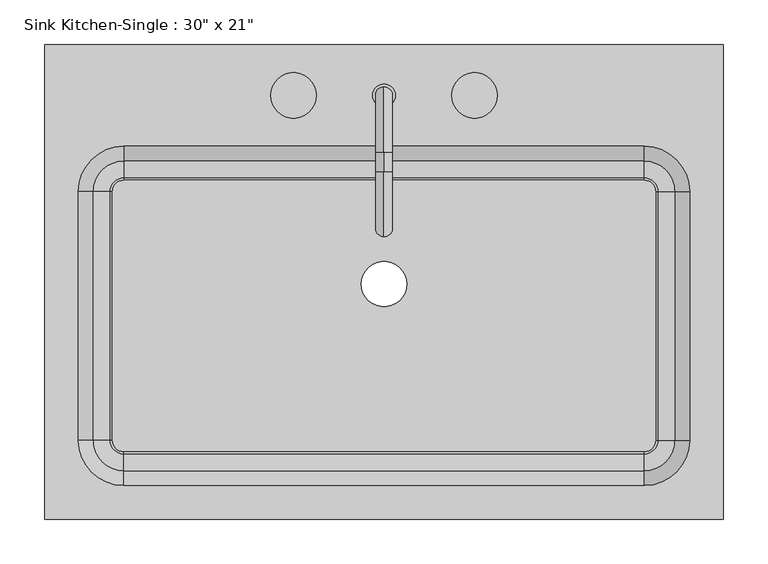
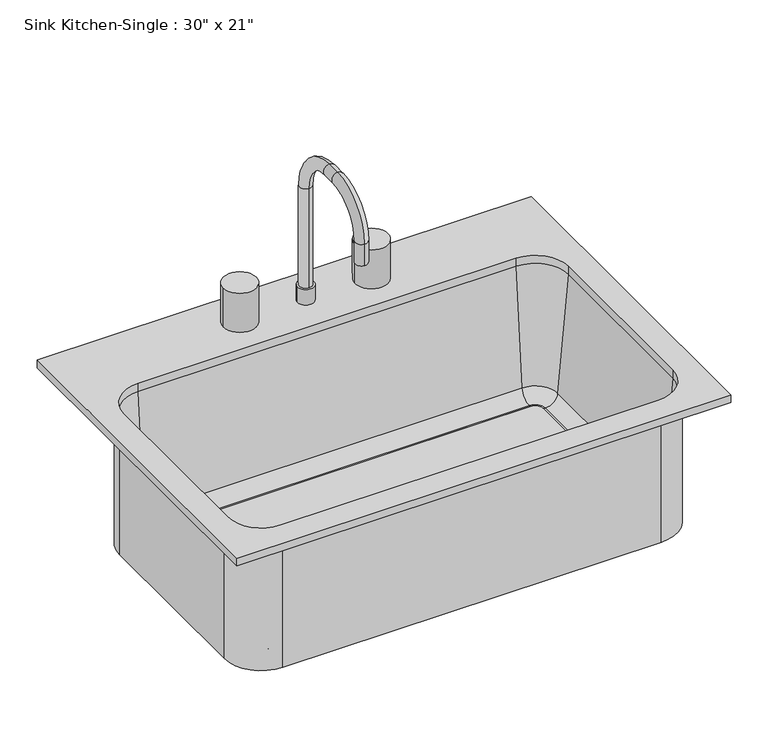
"""IFC4 building model written with IfcOpenShell, lengths in millimetres: flow terminal geometry."""

from ifc_helpers import new_model, si_unit, point, frame, frame_2d, origin, place, context, project, spatial, polyline, circle_curve, ellipse_curve, trimmed, segment, composite_curve, outline, extrude, source, transform, mapped, element, save
from ifc_brep_helpers import plane_surface, cylinder_surface, revolved_surface, advanced_brep


def flow_terminal_4d548711(model_context):
    return source(origin(), model_context, "Body", "SolidModel", [
        extrude(outline(composite_curve([segment(trimmed(circle_curve(frame_2d((307.7892406, 103.9454011)), 12.7), [point((307.7892406, 116.6454011))], [point((320.4892406, 103.9454011))], False, "CARTESIAN"), True, "CONTINUOUS"), segment(polyline([(320.4892406, 103.9454011), (320.4892406, -175.4545989)]), True, "CONTINUOUS"), segment(trimmed(circle_curve(frame_2d((307.7892406, -175.4545989)), 12.7), [point((320.4892406, -175.4545989))], [point((307.7892406, -188.1545989))], False, "CARTESIAN"), True, "CONTINUOUS"), segment(polyline([(307.7892406, -188.1545989), (-276.4107594, -188.1545989)]), True, "CONTINUOUS"), segment(trimmed(circle_curve(frame_2d((-276.4107594, -175.4545989)), 12.7), [point((-276.4107594, -188.1545989))], [point((-289.1107594, -175.4545989))], False, "CARTESIAN"), True, "CONTINUOUS"), segment(polyline([(-289.1107594, -175.4545989), (-289.1107594, 103.9454011)]), True, "CONTINUOUS"), segment(trimmed(circle_curve(frame_2d((-276.4107594, 103.9454011)), 12.7), [point((-289.1107594, 103.9454011))], [point((-276.4107594, 116.6454011))], False, "CARTESIAN"), True, "CONTINUOUS"), segment(polyline([(-276.4107594, 116.6454011), (307.7892406, 116.6454011)]), True, "CONTINUOUS")], self_intersect=False), holes=[composite_curve([segment(trimmed(circle_curve(frame_2d((15.6892406, 0.0)), 25.4), [point((-9.7107594, 0.0))], [point((41.0892406, 0.0))], True, "CARTESIAN"), True, "CONTINUOUS"), segment(trimmed(circle_curve(frame_2d((15.6892406, 0.0)), 25.4), [point((41.0892406, 0.0))], [point((-9.7107594, 0.0))], True, "CARTESIAN"), True, "CONTINUOUS")], self_intersect=False)]), frame((0.0, 0.0, 698.5), z_axis=(0.0, 0.0, 1.0), x_axis=(1.0, 0.0, 0.0)), (0.0, 0.0, 1.0), 9.525),
        extrude(outline(composite_curve([segment(trimmed(circle_curve(frame_2d((-85.9107594, 211.8954011)), 25.4), [point((-111.3107594, 211.8954011))], [point((-60.5107594, 211.8954011))], False, "CARTESIAN"), True, "CONTINUOUS"), segment(trimmed(circle_curve(frame_2d((-85.9107594, 211.8954011)), 25.4), [point((-60.5107594, 211.8954011))], [point((-111.3107594, 211.8954011))], False, "CARTESIAN"), True, "CONTINUOUS")], self_intersect=False)), frame((0.0, 0.0, 927.1), z_axis=(0.0, 0.0, 1.0), x_axis=(1.0, 0.0, 0.0)), (0.0, 0.0, 1.0), 63.5),
        extrude(outline(composite_curve([segment(trimmed(circle_curve(frame_2d((117.2892406, 211.8954011)), 25.4), [point((91.8892406, 211.8954011))], [point((142.6892406, 211.8954011))], False, "CARTESIAN"), True, "CONTINUOUS"), segment(trimmed(circle_curve(frame_2d((117.2892406, 211.8954011)), 25.4), [point((142.6892406, 211.8954011))], [point((91.8892406, 211.8954011))], False, "CARTESIAN"), True, "CONTINUOUS")], self_intersect=False)), frame((0.0, 0.0, 927.1), z_axis=(0.0, 0.0, 1.0), x_axis=(1.0, 0.0, 0.0)), (0.0, 0.0, 1.0), 63.5),
        advanced_brep(
        [(2.9892406, 211.8954011, 927.1), (28.3892406, 211.8954011, 927.1), (15.6892406, 221.4204011, 1114.425), (15.6892406, 202.3704011, 1114.425), (15.6892406, 202.3704011, 952.5), (15.6892406, 221.4204011, 952.5), (15.6892406, 148.3954011, 1187.45), (15.6892406, 148.3954011, 1168.4), (15.6892406, 126.1704011, 1187.45), (15.6892406, 126.1704011, 1168.4), (15.6892406, 53.1454011, 1114.425), (15.6892406, 72.1954011, 1114.425), (15.6892406, 53.1454011, 1079.5), (15.6892406, 72.1954011, 1079.5), (2.9892406, 211.8954011, 952.5), (28.3892406, 211.8954011, 952.5)],
        [
            (0, 1, circle_curve(frame((15.6892406, 211.8954011, 927.1), z_axis=(0.0, 0.0, -1.0), x_axis=(1.0, 0.0, 0.0)), 12.7)),
            (1, 0, circle_curve(frame((15.6892406, 211.8954011, 927.1), z_axis=(0.0, 0.0, -1.0), x_axis=(1.0, 0.0, 0.0)), 12.7)),
            (2, 3, circle_curve(frame((15.6892406, 211.8954011, 1114.425), z_axis=(0.0, 0.0, -1.0), x_axis=(0.0, -1.0, 0.0)), 9.525)),
            (3, 4),
            (4, 5, circle_curve(frame((15.6892406, 211.8954011, 952.5), z_axis=(0.0, 0.0, 1.0), x_axis=(0.0, -1.0, 0.0)), 9.525)),
            (5, 2),
            (3, 2, circle_curve(frame((15.6892406, 211.8954011, 1114.425), z_axis=(0.0, 0.0, -1.0), x_axis=(0.0, -1.0, 0.0)), 9.525)),
            (5, 4, circle_curve(frame((15.6892406, 211.8954011, 952.5), z_axis=(0.0, 0.0, 1.0), x_axis=(0.0, -1.0, 0.0)), 9.525)),
            (2, 6, circle_curve(frame((15.6892406, 148.3954011, 1114.425), z_axis=(1.0, 0.0, 0.0), x_axis=(0.0, 1.0, 0.0)), 73.025)),
            (6, 7, circle_curve(frame((15.6892406, 148.3954011, 1177.925), z_axis=(0.0, 1.0, 0.0), x_axis=(0.0, 0.0, -1.0)), 9.525)),
            (7, 3, circle_curve(frame((15.6892406, 148.3954011, 1114.425), z_axis=(-1.0, 0.0, 0.0), x_axis=(0.0, 1.0, 0.0)), 53.975)),
            (7, 6, circle_curve(frame((15.6892406, 148.3954011, 1177.925), z_axis=(0.0, 1.0, 0.0), x_axis=(0.0, 0.0, -1.0)), 9.525)),
            (6, 8),
            (8, 9, circle_curve(frame((15.6892406, 126.1704011, 1177.925), z_axis=(0.0, 1.0, 0.0), x_axis=(0.0, 0.0, -1.0)), 9.525)),
            (9, 7),
            (9, 8, circle_curve(frame((15.6892406, 126.1704011, 1177.925), z_axis=(0.0, 1.0, 0.0), x_axis=(0.0, 0.0, -1.0)), 9.525)),
            (8, 10, circle_curve(frame((15.6892406, 126.1704011, 1114.425), z_axis=(1.0, 0.0, 0.0), x_axis=(0.0, 0.0, 1.0)), 73.025)),
            (10, 11, circle_curve(frame((15.6892406, 62.6704011, 1114.425), z_axis=(0.0, 0.0, 1.0), x_axis=(0.0, 1.0, 0.0)), 9.525)),
            (11, 9, circle_curve(frame((15.6892406, 126.1704011, 1114.425), z_axis=(-1.0, 0.0, 0.0), x_axis=(0.0, 0.0, 1.0)), 53.975)),
            (11, 10, circle_curve(frame((15.6892406, 62.6704011, 1114.425), z_axis=(0.0, 0.0, 1.0), x_axis=(0.0, 1.0, 0.0)), 9.525)),
            (12, 13, circle_curve(frame((15.6892406, 62.6704011, 1079.5), z_axis=(0.0, 0.0, -1.0), x_axis=(0.0, 1.0, 0.0)), 9.525)),
            (13, 12, circle_curve(frame((15.6892406, 62.6704011, 1079.5), z_axis=(0.0, 0.0, -1.0), x_axis=(0.0, 1.0, 0.0)), 9.525)),
            (10, 12),
            (13, 11),
            (14, 15, circle_curve(frame((15.6892406, 211.8954011, 952.5), z_axis=(0.0, 0.0, 1.0), x_axis=(1.0, 0.0, 0.0)), 12.7)),
            (15, 14, circle_curve(frame((15.6892406, 211.8954011, 952.5), z_axis=(0.0, 0.0, 1.0), x_axis=(1.0, 0.0, 0.0)), 12.7)),
            (14, 0),
            (1, 15),
        ],
        [
            plane_surface(frame((15.6892406, 202.3704011, 927.1), z_axis=(0.0, 0.0, -1.0), x_axis=(1.0, 0.0, 0.0))),
            cylinder_surface(frame((15.6892406, 211.8954011, 927.1), z_axis=(0.0, 0.0, -1.0), x_axis=(0.0, -1.0, 0.0)), 9.525),
            revolved_surface(trimmed(ellipse_curve(frame((15.6892406, 211.8954011, 1114.425), z_axis=(0.0, 0.0, -1.0), x_axis=(0.0, -1.0, 0.0)), 9.525, 9.525), [point((15.6892406, 221.4204011, 1114.425))], [point((15.6892406, 202.3704011, 1114.425))], True, "CARTESIAN"), (15.6892406, 148.3954011, 1114.425), (1.0, 0.0, 0.0)),
            revolved_surface(trimmed(ellipse_curve(frame((15.6892406, 211.8954011, 1114.425), z_axis=(0.0, 0.0, -1.0), x_axis=(0.0, -1.0, 0.0)), 9.525, 9.525), [point((15.6892406, 202.3704011, 1114.425))], [point((15.6892406, 221.4204011, 1114.425))], True, "CARTESIAN"), (15.6892406, 148.3954011, 1114.425), (1.0, 0.0, 0.0)),
            cylinder_surface(frame((15.6892406, 148.3954011, 1177.925), z_axis=(0.0, 1.0, 0.0), x_axis=(0.0, 0.0, -1.0)), 9.525),
            revolved_surface(trimmed(ellipse_curve(frame((15.6892406, 126.1704011, 1177.925), z_axis=(0.0, 1.0, 0.0), x_axis=(0.0, 0.0, -1.0)), 9.525, 9.525), [point((15.6892406, 126.1704011, 1187.45))], [point((15.6892406, 126.1704011, 1168.4))], True, "CARTESIAN"), (15.6892406, 126.1704011, 1114.425), (1.0, 0.0, 0.0)),
            revolved_surface(trimmed(ellipse_curve(frame((15.6892406, 126.1704011, 1177.925), z_axis=(0.0, 1.0, 0.0), x_axis=(0.0, 0.0, -1.0)), 9.525, 9.525), [point((15.6892406, 126.1704011, 1168.4))], [point((15.6892406, 126.1704011, 1187.45))], True, "CARTESIAN"), (15.6892406, 126.1704011, 1114.425), (1.0, 0.0, 0.0)),
            plane_surface(frame((15.6892406, 53.1454011, 1079.5), z_axis=(0.0, 0.0, -1.0), x_axis=(-1.0, 0.0, 0.0))),
            cylinder_surface(frame((15.6892406, 62.6704011, 1114.425), z_axis=(0.0, 0.0, 1.0), x_axis=(0.0, 1.0, 0.0)), 9.525),
            plane_surface(frame((28.3892406, 211.8954011, 952.5), z_axis=(0.0, 0.0, 1.0), x_axis=(0.0, 1.0, 0.0))),
            cylinder_surface(frame((15.6892406, 211.8954011, 927.1), z_axis=(0.0, 0.0, 1.0), x_axis=(1.0, 0.0, 0.0)), 12.7),
        ],
        [
            (0, [[1, 2]]),
            (1, [[3, 4, 5, 6]]),
            (1, [[7, -6, 8, -4]]),
            (2, [[-3, 9, 10, 11]]),
            (3, [[-7, -11, 12, -9]]),
            (4, [[-10, 13, 14, 15]]),
            (4, [[-12, -15, 16, -13]]),
            (5, [[-14, 17, 18, 19]]),
            (6, [[-16, -19, 20, -17]]),
            (7, [[21, 22]]),
            (8, [[-18, 23, -22, 24]]),
            (8, [[-20, -24, -21, -23]]),
            (9, [[25, 26], [-5, -8]]),
            (10, [[-25, 27, -2, 28]]),
            (10, [[-26, -28, -1, -27]]),
        ],
    ),
        advanced_brep(
        [(396.6892406, 269.0454011, 927.1), (-365.3107594, 269.0454011, 927.1), (-365.3107594, -264.3545989, 927.1), (396.6892406, -264.3545989, 927.1), (307.7892406, 154.7454011, 927.1), (358.5892406, 103.9454011, 927.1), (358.5892406, -175.4545989, 927.1), (307.7892406, -226.2545989, 927.1), (-276.4107594, -226.2545989, 927.1), (-327.2107594, -175.4545989, 927.1), (-327.2107594, 103.9454011, 927.1), (-276.4107594, 154.7454011, 927.1), (396.6892406, 269.0454011, 914.4), (396.6892406, -264.3545989, 914.4), (-365.3107594, -264.3545989, 914.4), (-365.3107594, 269.0454011, 914.4), (364.9392406, 103.9454011, 914.4), (307.7892406, 161.0954011, 914.4), (-276.4107594, 161.0954011, 914.4), (-333.5607594, 103.9454011, 914.4), (-333.5607594, -175.4545989, 914.4), (-276.4107594, -232.6045989, 914.4), (307.7892406, -232.6045989, 914.4), (364.9392406, -175.4545989, 914.4), (307.7892406, 154.7454011, 914.4), (358.5892406, 103.9454011, 914.4), (358.5892406, -175.4545989, 914.4), (307.7892406, -226.2545989, 914.4), (-276.4107594, -226.2545989, 914.4), (-327.2107594, -175.4545989, 914.4), (-327.2107594, 103.9454011, 914.4), (-276.4107594, 154.7454011, 914.4), (364.9392406, 103.9454011, 698.5), (307.7892406, 161.0954011, 698.5), (320.4892406, 103.9454011, 698.5), (307.7892406, 116.6454011, 698.5), (320.4892406, 103.9454011, 708.025), (307.7892406, 116.6454011, 708.025), (323.0776588, 103.9454011, 708.025), (307.7892406, 119.2338193, 708.025), (342.0551678, 103.9454011, 725.4146831), (307.7892406, 138.2113283, 725.4146831), (364.9392406, -175.4545989, 698.5), (320.4892406, -175.4545989, 698.5), (320.4892406, -175.4545989, 708.025), (323.0776588, -175.4545989, 708.025), (342.0551678, -175.4545989, 725.4146831), (307.7892406, -232.6045989, 698.5), (307.7892406, -188.1545989, 698.5), (307.7892406, -188.1545989, 708.025), (307.7892406, -190.7430171, 708.025), (307.7892406, -209.7205261, 725.4146831), (-276.4107594, -232.6045989, 698.5), (-276.4107594, -188.1545989, 698.5), (-276.4107594, -188.1545989, 708.025), (-276.4107594, -190.7430171, 708.025), (-276.4107594, -209.7205261, 725.4146831), (-333.5607594, -175.4545989, 698.5), (-289.1107594, -175.4545989, 698.5), (-289.1107594, -175.4545989, 708.025), (-291.6991776, -175.4545989, 708.025), (-310.6766866, -175.4545989, 725.4146831), (-333.5607594, 103.9454011, 698.5), (-289.1107594, 103.9454011, 698.5), (-289.1107594, 103.9454011, 708.025), (-291.6991776, 103.9454011, 708.025), (-310.6766866, 103.9454011, 725.4146831), (-276.4107594, 161.0954011, 698.5), (-276.4107594, 116.6454011, 698.5), (-276.4107594, 116.6454011, 708.025), (-276.4107594, 119.2338193, 708.025), (-276.4107594, 138.2113283, 725.4146831)],
        [
            (0, 1),
            (1, 2),
            (2, 3),
            (3, 0),
            (4, 5, circle_curve(frame((307.7892406, 103.9454011, 927.1), z_axis=(0.0, 0.0, -1.0), x_axis=(1.0, 0.0, 0.0)), 50.8)),
            (5, 6),
            (6, 7, circle_curve(frame((307.7892406, -175.4545989, 927.1), z_axis=(0.0, 0.0, -1.0), x_axis=(1.0, 0.0, 0.0)), 50.8)),
            (7, 8),
            (8, 9, circle_curve(frame((-276.4107594, -175.4545989, 927.1), z_axis=(0.0, 0.0, -1.0), x_axis=(1.0, 0.0, 0.0)), 50.8)),
            (9, 10),
            (10, 11, circle_curve(frame((-276.4107594, 103.9454011, 927.1), z_axis=(0.0, 0.0, -1.0), x_axis=(1.0, 0.0, 0.0)), 50.8)),
            (11, 4),
            (12, 13),
            (13, 14),
            (14, 15),
            (15, 12),
            (16, 17, circle_curve(frame((307.7892406, 103.9454011, 914.4), z_axis=(0.0, 0.0, 1.0), x_axis=(0.0, 1.0, 0.0)), 57.15)),
            (17, 18),
            (18, 19, circle_curve(frame((-276.4107594, 103.9454011, 914.4), z_axis=(0.0, 0.0, 1.0), x_axis=(-1.0, 0.0, 0.0)), 57.15)),
            (19, 20),
            (20, 21, circle_curve(frame((-276.4107594, -175.4545989, 914.4), z_axis=(0.0, 0.0, 1.0), x_axis=(0.0, -1.0, 0.0)), 57.15)),
            (21, 22),
            (22, 23, circle_curve(frame((307.7892406, -175.4545989, 914.4), z_axis=(0.0, 0.0, 1.0), x_axis=(1.0, 0.0, 0.0)), 57.15)),
            (23, 16),
            (0, 12),
            (15, 1),
            (14, 2),
            (13, 3),
            (4, 24),
            (24, 25, circle_curve(frame((307.7892406, 103.9454011, 914.4), z_axis=(0.0, 0.0, -1.0), x_axis=(1.0, 0.0, 0.0)), 50.8)),
            (25, 5),
            (25, 26),
            (26, 6),
            (26, 27, circle_curve(frame((307.7892406, -175.4545989, 914.4), z_axis=(0.0, 0.0, -1.0), x_axis=(1.0, 0.0, 0.0)), 50.8)),
            (27, 7),
            (27, 28),
            (28, 8),
            (28, 29, circle_curve(frame((-276.4107594, -175.4545989, 914.4), z_axis=(0.0, 0.0, -1.0), x_axis=(1.0, 0.0, 0.0)), 50.8)),
            (29, 9),
            (29, 30),
            (30, 10),
            (30, 31, circle_curve(frame((-276.4107594, 103.9454011, 914.4), z_axis=(0.0, 0.0, -1.0), x_axis=(1.0, 0.0, 0.0)), 50.8)),
            (31, 11),
            (31, 24),
            (32, 33, circle_curve(frame((307.7892406, 103.9454011, 698.5), z_axis=(0.0, 0.0, 1.0), x_axis=(0.0, 1.0, 0.0)), 57.15)),
            (33, 17),
            (16, 32),
            (32, 34),
            (34, 35, circle_curve(frame((307.7892406, 103.9454011, 698.5), z_axis=(0.0, 0.0, 1.0), x_axis=(0.0, 1.0, 0.0)), 12.7)),
            (35, 33),
            (34, 36),
            (36, 37, circle_curve(frame((307.7892406, 103.9454011, 708.025), z_axis=(0.0, 0.0, 1.0), x_axis=(0.0, 1.0, 0.0)), 12.7)),
            (37, 35),
            (36, 38),
            (38, 39, circle_curve(frame((307.7892406, 103.9454011, 708.025), z_axis=(0.0, 0.0, 1.0), x_axis=(0.0, 1.0, 0.0)), 15.2884182)),
            (39, 37),
            (38, 40, circle_curve(frame((323.0776588, 103.9454011, 727.075), z_axis=(0.0, -1.0, 0.0), x_axis=(1.0, 0.0, 0.0)), 19.05)),
            (40, 41, circle_curve(frame((307.7892406, 103.9454011, 725.4146831), z_axis=(0.0, 0.0, 1.0), x_axis=(0.0, 1.0, 0.0)), 34.2659272)),
            (41, 39, circle_curve(frame((307.7892406, 119.2338193, 727.075), z_axis=(-1.0, 0.0, 0.0), x_axis=(0.0, 1.0, 0.0)), 19.05)),
            (40, 25),
            (24, 41),
            (23, 42),
            (42, 32),
            (42, 43),
            (43, 34),
            (43, 44),
            (44, 36),
            (44, 45),
            (45, 38),
            (45, 46, circle_curve(frame((323.0776588, -175.4545989, 727.075), z_axis=(0.0, -1.0, 0.0), x_axis=(1.0, 0.0, 0.0)), 19.05)),
            (46, 40),
            (46, 26),
            (22, 47),
            (47, 42, circle_curve(frame((307.7892406, -175.4545989, 698.5), z_axis=(0.0, 0.0, 1.0), x_axis=(1.0, 0.0, 0.0)), 57.15)),
            (47, 48),
            (48, 43, circle_curve(frame((307.7892406, -175.4545989, 698.5), z_axis=(0.0, 0.0, 1.0), x_axis=(1.0, 0.0, 0.0)), 12.7)),
            (48, 49),
            (49, 44, circle_curve(frame((307.7892406, -175.4545989, 708.025), z_axis=(0.0, 0.0, 1.0), x_axis=(1.0, 0.0, 0.0)), 12.7)),
            (49, 50),
            (50, 45, circle_curve(frame((307.7892406, -175.4545989, 708.025), z_axis=(0.0, 0.0, 1.0), x_axis=(1.0, 0.0, 0.0)), 15.2884182)),
            (50, 51, circle_curve(frame((307.7892406, -190.7430171, 727.075), z_axis=(-1.0, 0.0, 0.0), x_axis=(0.0, -1.0, 0.0)), 19.05)),
            (51, 46, circle_curve(frame((307.7892406, -175.4545989, 725.4146831), z_axis=(0.0, 0.0, 1.0), x_axis=(1.0, 0.0, 0.0)), 34.2659272)),
            (51, 27),
            (21, 52),
            (52, 47),
            (52, 53),
            (53, 48),
            (53, 54),
            (54, 49),
            (54, 55),
            (55, 50),
            (55, 56, circle_curve(frame((-276.4107594, -190.7430171, 727.075), z_axis=(-1.0, 0.0, 0.0), x_axis=(0.0, -1.0, 0.0)), 19.05)),
            (56, 51),
            (56, 28),
            (20, 57),
            (57, 52, circle_curve(frame((-276.4107594, -175.4545989, 698.5), z_axis=(0.0, 0.0, 1.0), x_axis=(0.0, -1.0, 0.0)), 57.15)),
            (57, 58),
            (58, 53, circle_curve(frame((-276.4107594, -175.4545989, 698.5), z_axis=(0.0, 0.0, 1.0), x_axis=(0.0, -1.0, 0.0)), 12.7)),
            (58, 59),
            (59, 54, circle_curve(frame((-276.4107594, -175.4545989, 708.025), z_axis=(0.0, 0.0, 1.0), x_axis=(0.0, -1.0, 0.0)), 12.7)),
            (59, 60),
            (60, 55, circle_curve(frame((-276.4107594, -175.4545989, 708.025), z_axis=(0.0, 0.0, 1.0), x_axis=(0.0, -1.0, 0.0)), 15.2884182)),
            (60, 61, circle_curve(frame((-291.6991776, -175.4545989, 727.075), z_axis=(0.0, 1.0, 0.0), x_axis=(-1.0, 0.0, 0.0)), 19.05)),
            (61, 56, circle_curve(frame((-276.4107594, -175.4545989, 725.4146831), z_axis=(0.0, 0.0, 1.0), x_axis=(0.0, -1.0, 0.0)), 34.2659272)),
            (61, 29),
            (19, 62),
            (62, 57),
            (62, 63),
            (63, 58),
            (63, 64),
            (64, 59),
            (64, 65),
            (65, 60),
            (65, 66, circle_curve(frame((-291.6991776, 103.9454011, 727.075), z_axis=(0.0, 1.0, 0.0), x_axis=(-1.0, 0.0, 0.0)), 19.05)),
            (66, 61),
            (66, 30),
            (18, 67),
            (67, 62, circle_curve(frame((-276.4107594, 103.9454011, 698.5), z_axis=(0.0, 0.0, 1.0), x_axis=(-1.0, 0.0, 0.0)), 57.15)),
            (67, 68),
            (68, 63, circle_curve(frame((-276.4107594, 103.9454011, 698.5), z_axis=(0.0, 0.0, 1.0), x_axis=(-1.0, 0.0, 0.0)), 12.7)),
            (68, 69),
            (69, 64, circle_curve(frame((-276.4107594, 103.9454011, 708.025), z_axis=(0.0, 0.0, 1.0), x_axis=(-1.0, 0.0, 0.0)), 12.7)),
            (69, 70),
            (70, 65, circle_curve(frame((-276.4107594, 103.9454011, 708.025), z_axis=(0.0, 0.0, 1.0), x_axis=(-1.0, 0.0, 0.0)), 15.2884182)),
            (70, 71, circle_curve(frame((-276.4107594, 119.2338193, 727.075), z_axis=(1.0, 0.0, 0.0), x_axis=(0.0, 1.0, 0.0)), 19.05)),
            (71, 66, circle_curve(frame((-276.4107594, 103.9454011, 725.4146831), z_axis=(0.0, 0.0, 1.0), x_axis=(-1.0, 0.0, 0.0)), 34.2659272)),
            (71, 31),
            (33, 67),
            (35, 68),
            (37, 69),
            (39, 70),
            (41, 71),
        ],
        [
            plane_surface(frame((-365.3107594, 269.0454011, 927.1), z_axis=(0.0, 0.0, 1.0), x_axis=(-1.0, 0.0, 0.0))),
            plane_surface(frame((-365.3107594, 269.0454011, 914.4), z_axis=(0.0, 0.0, -1.0), x_axis=(1.0, 0.0, 0.0))),
            plane_surface(frame((396.6892406, 269.0454011, 927.1), z_axis=(0.0, 1.0, 0.0), x_axis=(0.0, 0.0, -1.0))),
            plane_surface(frame((-365.3107594, 269.0454011, 927.1), z_axis=(-1.0, 0.0, 0.0), x_axis=(0.0, 0.0, -1.0))),
            plane_surface(frame((-365.3107594, -264.3545989, 927.1), z_axis=(0.0, -1.0, 0.0), x_axis=(0.0, 0.0, -1.0))),
            plane_surface(frame((396.6892406, -264.3545989, 927.1), z_axis=(1.0, 0.0, 0.0), x_axis=(0.0, 0.0, -1.0))),
            revolved_surface(polyline([(358.58924060000004, 103.9454011, 914.4), (358.58924060000004, 103.9454011, 927.1)]), (307.7892406, 103.9454011, 0.0), (0.0, 0.0, -1.0)),
            plane_surface(frame((358.5892406, 103.9454011, 927.1), z_axis=(-1.0, 0.0, 0.0), x_axis=(0.0, 0.0, -1.0))),
            revolved_surface(polyline([(358.58924060000004, -175.4545989, 914.4), (358.58924060000004, -175.4545989, 927.1)]), (307.7892406, -175.4545989, 0.0), (0.0, 0.0, -1.0)),
            plane_surface(frame((307.7892406, -226.2545989, 927.1), z_axis=(0.0, 1.0, 0.0), x_axis=(0.0, 0.0, -1.0))),
            revolved_surface(polyline([(-225.6107594, -175.4545989, 914.4), (-225.6107594, -175.4545989, 927.1)]), (-276.4107594, -175.4545989, 0.0), (0.0, 0.0, -1.0)),
            plane_surface(frame((-327.2107594, -175.4545989, 927.1), z_axis=(1.0, 0.0, 0.0), x_axis=(0.0, 0.0, -1.0))),
            revolved_surface(polyline([(-225.6107594, 103.9454011, 914.4), (-225.6107594, 103.9454011, 927.1)]), (-276.4107594, 103.9454011, 0.0), (0.0, 0.0, -1.0)),
            plane_surface(frame((-276.4107594, 154.7454011, 927.1), z_axis=(0.0, -1.0, 0.0), x_axis=(0.0, 0.0, -1.0))),
            cylinder_surface(frame((307.7892406, 103.9454011, 0.0), z_axis=(0.0, 0.0, -1.0), x_axis=(0.0, 1.0, 0.0)), 57.15),
            plane_surface(frame((307.7892406, 103.9454011, 698.5), z_axis=(0.0, 0.0, -1.0), x_axis=(0.0, 1.0, 0.0))),
            revolved_surface(polyline([(307.7892406, 116.6454011, 698.5), (307.7892406, 116.6454011, 708.025)]), (307.7892406, 103.9454011, 0.0), (0.0, 0.0, -1.0)),
            plane_surface(frame((307.7892406, 103.9454011, 708.025), z_axis=(0.0, 0.0, 1.0), x_axis=(0.0, 1.0, 0.0))),
            revolved_surface(trimmed(ellipse_curve(frame((307.7892406, 119.2338193, 727.075), z_axis=(1.0, 0.0, 0.0), x_axis=(0.0, 1.0, 0.0)), 19.05, 19.05), [point((307.7892406, 119.2338193, 708.025))], [point((307.7892406, 138.2113283, 725.4146831))], True, "CARTESIAN"), (307.7892406, 103.9454011, 0.0), (0.0, 0.0, -1.0)),
            revolved_surface(polyline([(307.7892406, 138.2113283, 725.4146831), (307.7892406, 154.7454011, 914.4)]), (307.7892406, 103.9454011, 0.0), (0.0, 0.0, -1.0)),
            plane_surface(frame((364.9392406, 103.9454011, 914.4), z_axis=(1.0, 0.0, 0.0), x_axis=(0.0, -1.0, 0.0))),
            plane_surface(frame((364.9392406, 103.9454011, 698.5), z_axis=(0.0, 0.0, -1.0), x_axis=(0.0, -1.0, 0.0))),
            plane_surface(frame((320.4892406, 103.9454011, 698.5), z_axis=(-1.0, 0.0, 0.0), x_axis=(0.0, -1.0, 0.0))),
            plane_surface(frame((320.4892406, 103.9454011, 708.025), z_axis=(0.0, 0.0, 1.0), x_axis=(0.0, -1.0, 0.0))),
            revolved_surface(polyline([(342.1276588, -175.45459889999998, 727.075), (342.1276588, 103.9454011, 727.075)]), (323.0776588, 103.9454011, 727.075), (0.0, -1.0, 0.0)),
            plane_surface(frame((342.0551678, 103.9454011, 725.4146831), z_axis=(-0.9961946980917442, 0.0, 0.08715574274767306), x_axis=(0.0, -1.0, 0.0))),
            cylinder_surface(frame((307.7892406, -175.4545989, 0.0), z_axis=(0.0, 0.0, -1.0), x_axis=(1.0, 0.0, 0.0)), 57.15),
            plane_surface(frame((307.7892406, -175.4545989, 698.5), z_axis=(0.0, 0.0, -1.0), x_axis=(1.0, 0.0, 0.0))),
            revolved_surface(polyline([(320.4892406, -175.4545989, 698.5), (320.4892406, -175.4545989, 708.025)]), (307.7892406, -175.4545989, 0.0), (0.0, 0.0, -1.0)),
            plane_surface(frame((307.7892406, -175.4545989, 708.025), z_axis=(0.0, 0.0, 1.0), x_axis=(1.0, 0.0, 0.0))),
            revolved_surface(trimmed(ellipse_curve(frame((323.0776588, -175.4545989, 727.075), z_axis=(0.0, -1.0, 0.0), x_axis=(1.0, 0.0, 0.0)), 19.05, 19.05), [point((323.0776588, -175.4545989, 708.025))], [point((342.0551678, -175.4545989, 725.4146831))], True, "CARTESIAN"), (307.7892406, -175.4545989, 0.0), (0.0, 0.0, -1.0)),
            revolved_surface(polyline([(342.0551678, -175.4545989, 725.4146831), (358.5892406, -175.4545989, 914.4)]), (307.7892406, -175.4545989, 0.0), (0.0, 0.0, -1.0)),
            plane_surface(frame((307.7892406, -232.6045989, 914.4), z_axis=(0.0, -1.0, 0.0), x_axis=(-1.0, 0.0, 0.0))),
            plane_surface(frame((307.7892406, -232.6045989, 698.5), z_axis=(0.0, 0.0, -1.0), x_axis=(-1.0, 0.0, 0.0))),
            plane_surface(frame((307.7892406, -188.1545989, 698.5), z_axis=(0.0, 1.0, 0.0), x_axis=(-1.0, 0.0, 0.0))),
            plane_surface(frame((307.7892406, -188.1545989, 708.025), z_axis=(0.0, 0.0, 1.0), x_axis=(-1.0, 0.0, 0.0))),
            revolved_surface(polyline([(-276.4107594, -209.79301710000001, 727.075), (307.7892406, -209.79301710000001, 727.075)]), (307.7892406, -190.7430171, 727.075), (-1.0, 0.0, 0.0)),
            plane_surface(frame((307.7892406, -209.7205261, 725.4146831), z_axis=(0.0, 0.9961946980917442, 0.08715574274767306), x_axis=(-1.0, 0.0, 0.0))),
            cylinder_surface(frame((-276.4107594, -175.4545989, 0.0), z_axis=(0.0, 0.0, -1.0), x_axis=(0.0, -1.0, 0.0)), 57.15),
            plane_surface(frame((-276.4107594, -175.4545989, 698.5), z_axis=(0.0, 0.0, -1.0), x_axis=(0.0, -1.0, 0.0))),
            revolved_surface(polyline([(-276.4107594, -188.1545989, 698.5), (-276.4107594, -188.1545989, 708.025)]), (-276.4107594, -175.4545989, 0.0), (0.0, 0.0, -1.0)),
            plane_surface(frame((-276.4107594, -175.4545989, 708.025), z_axis=(0.0, 0.0, 1.0), x_axis=(0.0, -1.0, 0.0))),
            revolved_surface(trimmed(ellipse_curve(frame((-276.4107594, -190.7430171, 727.075), z_axis=(-1.0, 0.0, 0.0), x_axis=(0.0, -1.0, 0.0)), 19.05, 19.05), [point((-276.4107594, -190.7430171, 708.025))], [point((-276.4107594, -209.7205261, 725.4146831))], True, "CARTESIAN"), (-276.4107594, -175.4545989, 0.0), (0.0, 0.0, -1.0)),
            revolved_surface(polyline([(-276.4107594, -209.7205261, 725.4146831), (-276.4107594, -226.2545989, 914.4)]), (-276.4107594, -175.4545989, 0.0), (0.0, 0.0, -1.0)),
            plane_surface(frame((-333.5607594, -175.4545989, 914.4), z_axis=(-1.0, 0.0, 0.0), x_axis=(0.0, 1.0, 0.0))),
            plane_surface(frame((-333.5607594, -175.4545989, 698.5), z_axis=(0.0, 0.0, -1.0), x_axis=(0.0, 1.0, 0.0))),
            plane_surface(frame((-289.1107594, -175.4545989, 698.5), z_axis=(1.0, 0.0, 0.0), x_axis=(0.0, 1.0, 0.0))),
            plane_surface(frame((-289.1107594, -175.4545989, 708.025), z_axis=(0.0, 0.0, 1.0), x_axis=(0.0, 1.0, 0.0))),
            revolved_surface(polyline([(-310.7491776, 103.94540109999997, 727.075), (-310.7491776, -175.4545989, 727.075)]), (-291.6991776, -175.4545989, 727.075), (0.0, 1.0, 0.0)),
            plane_surface(frame((-310.6766866, -175.4545989, 725.4146831), z_axis=(0.9961946980917442, 0.0, 0.08715574274767306), x_axis=(0.0, 1.0, 0.0))),
            cylinder_surface(frame((-276.4107594, 103.9454011, 0.0), z_axis=(0.0, 0.0, -1.0), x_axis=(-1.0, 0.0, 0.0)), 57.15),
            plane_surface(frame((-276.4107594, 103.9454011, 698.5), z_axis=(0.0, 0.0, -1.0), x_axis=(-1.0, 0.0, 0.0))),
            revolved_surface(polyline([(-289.1107594, 103.9454011, 698.5), (-289.1107594, 103.9454011, 708.025)]), (-276.4107594, 103.9454011, 0.0), (0.0, 0.0, -1.0)),
            plane_surface(frame((-276.4107594, 103.9454011, 708.025), z_axis=(0.0, 0.0, 1.0), x_axis=(-1.0, 0.0, 0.0))),
            revolved_surface(trimmed(ellipse_curve(frame((-291.6991776, 103.9454011, 727.075), z_axis=(0.0, 1.0, 0.0), x_axis=(-1.0, 0.0, 0.0)), 19.05, 19.05), [point((-291.6991776, 103.9454011, 708.025))], [point((-310.6766866, 103.9454011, 725.4146831))], True, "CARTESIAN"), (-276.4107594, 103.9454011, 0.0), (0.0, 0.0, -1.0)),
            revolved_surface(polyline([(-310.6766866, 103.9454011, 725.4146831), (-327.2107594, 103.9454011, 914.4)]), (-276.4107594, 103.9454011, 0.0), (0.0, 0.0, -1.0)),
            plane_surface(frame((-276.4107594, 161.0954011, 914.4), z_axis=(0.0, 1.0, 0.0), x_axis=(1.0, 0.0, 0.0))),
            plane_surface(frame((-276.4107594, 161.0954011, 698.5), z_axis=(0.0, 0.0, -1.0), x_axis=(1.0, 0.0, 0.0))),
            plane_surface(frame((-276.4107594, 116.6454011, 698.5), z_axis=(0.0, -1.0, 0.0), x_axis=(1.0, 0.0, 0.0))),
            plane_surface(frame((-276.4107594, 116.6454011, 708.025), z_axis=(0.0, 0.0, 1.0), x_axis=(1.0, 0.0, 0.0))),
            revolved_surface(polyline([(307.7892406, 138.2838193, 727.075), (-276.4107594, 138.2838193, 727.075)]), (-276.4107594, 119.2338193, 727.075), (1.0, 0.0, 0.0)),
            plane_surface(frame((-276.4107594, 138.2113283, 725.4146831), z_axis=(0.0, -0.9961946980917442, 0.08715574274767306), x_axis=(1.0, 0.0, 0.0))),
        ],
        [
            (0, [[1, 2, 3, 4], [5, 6, 7, 8, 9, 10, 11, 12]]),
            (1, [[13, 14, 15, 16], [17, 18, 19, 20, 21, 22, 23, 24]]),
            (2, [[-1, 25, -16, 26]]),
            (3, [[-2, -26, -15, 27]]),
            (4, [[-3, -27, -14, 28]]),
            (5, [[-4, -28, -13, -25]]),
            (6, [[-5, 29, 30, 31]]),
            (7, [[-6, -31, 32, 33]]),
            (8, [[-7, -33, 34, 35]]),
            (9, [[-8, -35, 36, 37]]),
            (10, [[-9, -37, 38, 39]]),
            (11, [[-10, -39, 40, 41]]),
            (12, [[-11, -41, 42, 43]]),
            (13, [[-12, -43, 44, -29]]),
            (14, [[45, 46, -17, 47]]),
            (15, [[-45, 48, 49, 50]]),
            (16, [[-49, 51, 52, 53]]),
            (17, [[-52, 54, 55, 56]]),
            (18, [[-55, 57, 58, 59]]),
            (19, [[-58, 60, -30, 61]]),
            (20, [[-47, -24, 62, 63]]),
            (21, [[-48, -63, 64, 65]]),
            (22, [[-51, -65, 66, 67]]),
            (23, [[-54, -67, 68, 69]]),
            (24, [[-57, -69, 70, 71]]),
            (25, [[-60, -71, 72, -32]]),
            (26, [[-62, -23, 73, 74]]),
            (27, [[-64, -74, 75, 76]]),
            (28, [[-66, -76, 77, 78]]),
            (29, [[-68, -78, 79, 80]]),
            (30, [[-70, -80, 81, 82]]),
            (31, [[-72, -82, 83, -34]]),
            (32, [[-73, -22, 84, 85]]),
            (33, [[-75, -85, 86, 87]]),
            (34, [[-77, -87, 88, 89]]),
            (35, [[-79, -89, 90, 91]]),
            (36, [[-81, -91, 92, 93]]),
            (37, [[-83, -93, 94, -36]]),
            (38, [[-84, -21, 95, 96]]),
            (39, [[-86, -96, 97, 98]]),
            (40, [[-88, -98, 99, 100]]),
            (41, [[-90, -100, 101, 102]]),
            (42, [[-92, -102, 103, 104]]),
            (43, [[-94, -104, 105, -38]]),
            (44, [[-95, -20, 106, 107]]),
            (45, [[-97, -107, 108, 109]]),
            (46, [[-99, -109, 110, 111]]),
            (47, [[-101, -111, 112, 113]]),
            (48, [[-103, -113, 114, 115]]),
            (49, [[-105, -115, 116, -40]]),
            (50, [[-106, -19, 117, 118]]),
            (51, [[-108, -118, 119, 120]]),
            (52, [[-110, -120, 121, 122]]),
            (53, [[-112, -122, 123, 124]]),
            (54, [[-114, -124, 125, 126]]),
            (55, [[-116, -126, 127, -42]]),
            (56, [[-46, 128, -117, -18]]),
            (57, [[-50, 129, -119, -128]]),
            (58, [[-53, 130, -121, -129]]),
            (59, [[-56, 131, -123, -130]]),
            (60, [[-59, 132, -125, -131]]),
            (61, [[-61, -44, -127, -132]]),
        ],
    ),
    ])


if __name__ == "__main__":
    model = new_model("IFC4")
    model_context = context("Model", 3, world=origin())
    ifc_project = project(units=[si_unit("LENGTHUNIT", "METRE", prefix="MILLI")], contexts=[model_context])
    site = spatial("IfcSite", under=ifc_project)
    building = spatial("IfcBuilding", under=site)
    placement = place(None, origin())
    flow_terminal_shape = flow_terminal_4d548711(model_context)
    element("IfcFlowTerminal", 1, ObjectType="Sink Kitchen-Single : 30\" x 21\"", at=placement, inside=building, context=model_context, shape_type="MappedRepresentation", body=[
        mapped(flow_terminal_shape, transform((0.0, 0.0, 0.0), x_axis=(1.0, 0.0, 0.0), y_axis=(0.0, 1.0, 0.0), z_axis=(0.0, 0.0, 1.0))),
    ])
    save(model, "model.ifc")

# Revit data of these elements
# Type "Sink Kitchen-Single : 30\" x 21\""
#   Assembly Code = "D2010410"
#   Counter Height = 3 ft
#   Depth = 1.75 ft
#   Width = 2.5 ft
#   Faucet Material = Steel, Polished
#   Sink Material = Steel, Polished
#   Default Elevation = 0
# Element 1 (IfcFlowTerminal, "Sink Kitchen-Single : 30\" x 21\"")
#   Materials on its faces: "Steel, Polished"
# Materials
#   "Steel, Polished": class "Metal", colour RGB 57 57 57, transparency 0, Description = "Polished steel", Cost = 0
